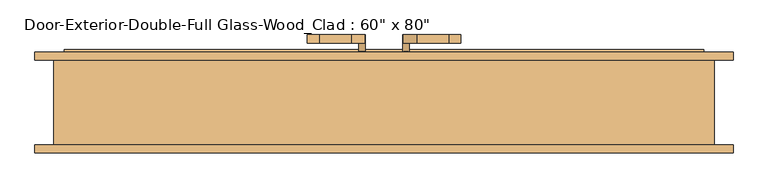
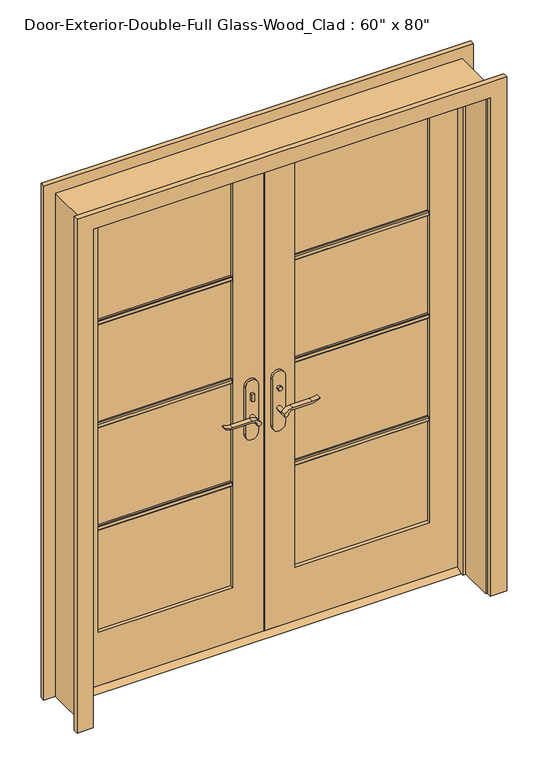
"""IFC4 building model written with IfcOpenShell, lengths in millimetres: door geometry."""

from ifc_helpers import new_model, si_unit, point, frame, frame_2d, origin, place, context, project, spatial, polyline, circle_curve, trimmed, segment, composite_curve, outline, extrude, faceted_brep, source, transform, mapped, element, save


def door_b03bd389(model_context):
    return source(origin(), model_context, "Body", "SolidModel", [
        extrude(outline(polyline([(63.5, 12.7), (98.425, 12.7), (123.825, 0.0), (38.1, 0.0), (63.5, 12.7)])), frame((-762.0, 0.0, 0.0), z_axis=(1.0, 0.0, 0.0), x_axis=(0.0, 1.0, 0.0)), (0.0, 0.0, 1.0), 1524.0),
        extrude(outline(polyline([(-47.4019111, 43.5), (-57.4019111, 43.5), (-57.4019111, 53.5), (-47.4019111, 53.5), (-47.4019111, 43.5)])), frame((0.0, 0.0, 981.9), z_axis=(0.0, 0.0, 1.0), x_axis=(1.0, 0.0, 0.0)), (0.0, 0.0, 1.0), 30.0),
        extrude(outline(composite_curve([segment(trimmed(circle_curve(frame_2d((996.9, -52.4019111)), 8.0), [point((996.9, -60.4019111))], [point((996.9, -44.4019111))], False, "CARTESIAN"), True, "CONTINUOUS"), segment(trimmed(circle_curve(frame_2d((996.9, -52.4019111)), 8.0), [point((996.9, -44.4019111))], [point((996.9, -60.4019111))], False, "CARTESIAN"), True, "CONTINUOUS")], self_intersect=False)), frame((0.0, 108.425, 0.0), z_axis=(0.0, 1.0, 0.0), x_axis=(0.0, 0.0, 1.0)), (0.0, 0.0, 1.0), 10.0),
        extrude(outline(composite_curve([segment(trimmed(circle_curve(frame_2d((897.1555521, -76.0694241)), 37.2832219), [point((919.0523287, -45.8937749))], [point((934.4, -77.7693445))], False, "CARTESIAN"), True, "CONTINUOUS"), segment(polyline([(934.4, -77.7693445), (934.4, -154.045502)]), True, "CONTINUOUS"), segment(trimmed(circle_curve(frame_2d((1017.6850638, -153.9791202)), 83.2850902), [point((934.4, -154.045502))], [point((939.4, -182.4019111))], True, "CARTESIAN"), True, "CONTINUOUS"), segment(polyline([(939.4, -182.4019111), (936.6135558, -182.4019111)]), True, "CONTINUOUS"), segment(trimmed(circle_curve(frame_2d((986.6709207, -150.4622499)), 59.3791355), [point((936.6135558, -182.4019111))], [point((927.4, -154.045502))], False, "CARTESIAN"), True, "CONTINUOUS"), segment(polyline([(927.4, -154.045502), (927.4, -77.7881013)]), True, "CONTINUOUS"), segment(trimmed(circle_curve(frame_2d((909.2738613, -77.7881013)), 18.1261387), [point((927.4, -77.7881013))], [point((914.4, -60.4019111))], True, "CARTESIAN"), True, "CONTINUOUS"), segment(trimmed(circle_curve(frame_2d((914.4, -52.4019111)), 8.0), [point((914.4, -60.4019111))], [point((919.0523287, -45.8937749))], False, "CARTESIAN"), True, "CONTINUOUS")], self_intersect=False)), frame((0.0, 3.5, 0.0), z_axis=(0.0, 1.0, 0.0), x_axis=(0.0, 0.0, 1.0)), (0.0, 0.0, 1.0), 20.0),
        extrude(outline(composite_curve([segment(trimmed(circle_curve(frame_2d((914.4, -52.4019111)), 8.0), [point((914.3999903, -60.4019111))], [point((919.0523287, -45.8937749))], False, "CARTESIAN"), True, "CONTINUOUS"), segment(trimmed(circle_curve(frame_2d((897.1555521, -76.0694241)), 37.2832219), [point((919.0523287, -45.8937749))], [point((934.4, -77.7693445))], False, "CARTESIAN"), True, "CONTINUOUS"), segment(polyline([(934.4, -77.7693445), (934.4, -154.045502)]), True, "CONTINUOUS"), segment(trimmed(circle_curve(frame_2d((1017.6850638, -153.9791202)), 83.2850902), [point((934.4, -154.045502))], [point((939.4, -182.4019111))], True, "CARTESIAN"), True, "CONTINUOUS"), segment(polyline([(939.4, -182.4019111), (936.6135558, -182.4019111)]), True, "CONTINUOUS"), segment(trimmed(circle_curve(frame_2d((986.6709207, -150.4622499)), 59.3791355), [point((936.6135558, -182.4019111))], [point((927.4, -154.045502))], False, "CARTESIAN"), True, "CONTINUOUS"), segment(polyline([(927.4, -154.045502), (927.4, -77.788099)]), True, "CONTINUOUS"), segment(trimmed(circle_curve(frame_2d((909.2738682, -77.788099)), 18.1261318), [point((927.4, -77.788099))], [point((914.3999903, -60.4019111))], True, "CARTESIAN"), True, "CONTINUOUS")], self_intersect=False)), frame((0.0, 138.425, 0.0), z_axis=(0.0, 1.0, 0.0), x_axis=(0.0, 0.0, 1.0)), (0.0, 0.0, 1.0), 20.0),
        extrude(outline(composite_curve([segment(trimmed(circle_curve(frame_2d((914.4, -52.4019111)), 8.0), [point((914.4, -60.4019111))], [point((914.4, -44.4019111))], False, "CARTESIAN"), True, "CONTINUOUS"), segment(trimmed(circle_curve(frame_2d((914.4, -52.4019111)), 8.0), [point((914.4, -44.4019111))], [point((914.4, -60.4019111))], False, "CARTESIAN"), True, "CONTINUOUS")], self_intersect=False)), frame((0.0, 23.5, 0.0), z_axis=(0.0, 1.0, 0.0), x_axis=(0.0, 0.0, 1.0)), (0.0, 0.0, 1.0), 30.0),
        extrude(outline(composite_curve([segment(trimmed(circle_curve(frame_2d((914.4, -52.4019111)), 8.0), [point((914.4, -60.4019111))], [point((914.4, -44.4019111))], False, "CARTESIAN"), True, "CONTINUOUS"), segment(trimmed(circle_curve(frame_2d((914.4, -52.4019111)), 8.0), [point((914.4, -44.4019111))], [point((914.4, -60.4019111))], False, "CARTESIAN"), True, "CONTINUOUS")], self_intersect=False)), frame((0.0, 108.425, 0.0), z_axis=(0.0, 1.0, 0.0), x_axis=(0.0, 0.0, 1.0)), (0.0, 0.0, 1.0), 30.0),
        extrude(outline(composite_curve([segment(polyline([(844.4, -27.4019111), (1039.4, -27.4019111)]), True, "CONTINUOUS"), segment(trimmed(circle_curve(frame_2d((1039.4, -52.4019111)), 25.0), [point((1039.4, -27.4019111))], [point((1039.4, -77.4019111))], False, "CARTESIAN"), True, "CONTINUOUS"), segment(polyline([(1039.4, -77.4019111), (844.4, -77.4019111)]), True, "CONTINUOUS"), segment(trimmed(circle_curve(frame_2d((844.4, -52.4019111)), 25.0), [point((844.4, -77.4019111))], [point((844.4, -27.4019111))], False, "CARTESIAN"), True, "CONTINUOUS")], self_intersect=False)), frame((0.0, 53.5, 0.0), z_axis=(0.0, 1.0, 0.0), x_axis=(0.0, 0.0, 1.0)), (0.0, 0.0, 1.0), 10.0),
        extrude(outline(composite_curve([segment(polyline([(844.4, -27.4019111), (1039.4, -27.4019111)]), True, "CONTINUOUS"), segment(trimmed(circle_curve(frame_2d((1039.4, -52.4019111)), 25.0), [point((1039.4, -27.4019111))], [point((1039.4, -77.4019111))], False, "CARTESIAN"), True, "CONTINUOUS"), segment(polyline([(1039.4, -77.4019111), (844.4, -77.4019111)]), True, "CONTINUOUS"), segment(trimmed(circle_curve(frame_2d((844.4, -52.4019111)), 25.0), [point((844.4, -77.4019111))], [point((844.4, -27.4019111))], False, "CARTESIAN"), True, "CONTINUOUS")], self_intersect=False)), frame((0.0, 98.425, 0.0), z_axis=(0.0, 1.0, 0.0), x_axis=(0.0, 0.0, 1.0)), (0.0, 0.0, 1.0), 10.0),
        extrude(outline(polyline([(47.3875, 118.425), (57.3875, 118.425), (57.3875, 108.425), (47.3875, 108.425), (47.3875, 118.425)])), frame((0.0, 0.0, 981.9), z_axis=(0.0, 0.0, 1.0), x_axis=(1.0, 0.0, 0.0)), (0.0, 0.0, 1.0), 30.0),
        extrude(outline(composite_curve([segment(trimmed(circle_curve(frame_2d((996.9, 52.3875)), 8.0), [point((996.9, 60.3875))], [point((996.9, 44.3875))], False, "CARTESIAN"), True, "CONTINUOUS"), segment(trimmed(circle_curve(frame_2d((996.9, 52.3875)), 8.0), [point((996.9, 44.3875))], [point((996.9, 60.3875))], False, "CARTESIAN"), True, "CONTINUOUS")], self_intersect=False)), frame((0.0, 43.5, 0.0), z_axis=(0.0, 1.0, 0.0), x_axis=(0.0, 0.0, 1.0)), (0.0, 0.0, 1.0), 10.0),
        extrude(outline(composite_curve([segment(trimmed(circle_curve(frame_2d((914.4, 52.3875)), 8.0), [point((919.0523287, 45.8793637))], [point((914.4, 60.3875))], False, "CARTESIAN"), True, "CONTINUOUS"), segment(trimmed(circle_curve(frame_2d((909.2738613, 77.7736901)), 18.1261387), [point((914.4, 60.3875))], [point((927.4, 77.7736901))], True, "CARTESIAN"), True, "CONTINUOUS"), segment(polyline([(927.4, 77.7736901), (927.4, 154.0310909)]), True, "CONTINUOUS"), segment(trimmed(circle_curve(frame_2d((986.6709207, 150.4478388)), 59.3791355), [point((927.4, 154.0310909))], [point((936.6135558, 182.3875))], False, "CARTESIAN"), True, "CONTINUOUS"), segment(polyline([(936.6135558, 182.3875), (939.4, 182.3875)]), True, "CONTINUOUS"), segment(trimmed(circle_curve(frame_2d((1017.6850638, 153.9647091)), 83.2850902), [point((939.4, 182.3875))], [point((934.4, 154.0310909))], True, "CARTESIAN"), True, "CONTINUOUS"), segment(polyline([(934.4, 154.0310909), (934.4, 77.7549333)]), True, "CONTINUOUS"), segment(trimmed(circle_curve(frame_2d((897.1555521, 76.0550129)), 37.2832219), [point((934.4, 77.7549333))], [point((919.0523287, 45.8793637))], False, "CARTESIAN"), True, "CONTINUOUS")], self_intersect=False)), frame((0.0, 138.425, 0.0), z_axis=(0.0, 1.0, 0.0), x_axis=(0.0, 0.0, 1.0)), (0.0, 0.0, 1.0), 20.0),
        extrude(outline(composite_curve([segment(trimmed(circle_curve(frame_2d((909.2738682, 77.7736878)), 18.1261318), [point((914.3999903, 60.3875))], [point((927.4, 77.7736878))], True, "CARTESIAN"), True, "CONTINUOUS"), segment(polyline([(927.4, 77.7736878), (927.4, 154.0310909)]), True, "CONTINUOUS"), segment(trimmed(circle_curve(frame_2d((986.6709207, 150.4478388)), 59.3791355), [point((927.4, 154.0310909))], [point((936.6135558, 182.3875))], False, "CARTESIAN"), True, "CONTINUOUS"), segment(polyline([(936.6135558, 182.3875), (939.4, 182.3875)]), True, "CONTINUOUS"), segment(trimmed(circle_curve(frame_2d((1017.6850638, 153.9647091)), 83.2850902), [point((939.4, 182.3875))], [point((934.4, 154.0310909))], True, "CARTESIAN"), True, "CONTINUOUS"), segment(polyline([(934.4, 154.0310909), (934.4, 77.7549333)]), True, "CONTINUOUS"), segment(trimmed(circle_curve(frame_2d((897.1555521, 76.0550129)), 37.2832219), [point((934.4, 77.7549333))], [point((919.0523287, 45.8793637))], False, "CARTESIAN"), True, "CONTINUOUS"), segment(trimmed(circle_curve(frame_2d((914.4, 52.3875)), 8.0), [point((919.0523287, 45.8793637))], [point((914.3999903, 60.3875))], False, "CARTESIAN"), True, "CONTINUOUS")], self_intersect=False)), frame((0.0, 3.5, 0.0), z_axis=(0.0, 1.0, 0.0), x_axis=(0.0, 0.0, 1.0)), (0.0, 0.0, 1.0), 20.0),
        extrude(outline(composite_curve([segment(trimmed(circle_curve(frame_2d((914.4, 52.3875)), 8.0), [point((914.4, 60.3875))], [point((914.4, 44.3875))], False, "CARTESIAN"), True, "CONTINUOUS"), segment(trimmed(circle_curve(frame_2d((914.4, 52.3875)), 8.0), [point((914.4, 44.3875))], [point((914.4, 60.3875))], False, "CARTESIAN"), True, "CONTINUOUS")], self_intersect=False)), frame((0.0, 108.425, 0.0), z_axis=(0.0, 1.0, 0.0), x_axis=(0.0, 0.0, 1.0)), (0.0, 0.0, 1.0), 30.0),
        extrude(outline(composite_curve([segment(trimmed(circle_curve(frame_2d((914.4, 52.3875)), 8.0), [point((914.4, 60.3875))], [point((914.4, 44.3875))], False, "CARTESIAN"), True, "CONTINUOUS"), segment(trimmed(circle_curve(frame_2d((914.4, 52.3875)), 8.0), [point((914.4, 44.3875))], [point((914.4, 60.3875))], False, "CARTESIAN"), True, "CONTINUOUS")], self_intersect=False)), frame((0.0, 23.5, 0.0), z_axis=(0.0, 1.0, 0.0), x_axis=(0.0, 0.0, 1.0)), (0.0, 0.0, 1.0), 30.0),
        extrude(outline(composite_curve([segment(trimmed(circle_curve(frame_2d((844.4, 52.3875)), 25.0), [point((844.4, 27.3875))], [point((844.4, 77.3875))], False, "CARTESIAN"), True, "CONTINUOUS"), segment(polyline([(844.4, 77.3875), (1039.4, 77.3875)]), True, "CONTINUOUS"), segment(trimmed(circle_curve(frame_2d((1039.4, 52.3875)), 25.0), [point((1039.4, 77.3875))], [point((1039.4, 27.3875))], False, "CARTESIAN"), True, "CONTINUOUS"), segment(polyline([(1039.4, 27.3875), (844.4, 27.3875)]), True, "CONTINUOUS")], self_intersect=False)), frame((0.0, 98.425, 0.0), z_axis=(0.0, 1.0, 0.0), x_axis=(0.0, 0.0, 1.0)), (0.0, 0.0, 1.0), 10.0),
        extrude(outline(composite_curve([segment(trimmed(circle_curve(frame_2d((844.4, 52.3875)), 25.0), [point((844.4, 27.3875))], [point((844.4, 77.3875))], False, "CARTESIAN"), True, "CONTINUOUS"), segment(polyline([(844.4, 77.3875), (1039.4, 77.3875)]), True, "CONTINUOUS"), segment(trimmed(circle_curve(frame_2d((1039.4, 52.3875)), 25.0), [point((1039.4, 77.3875))], [point((1039.4, 27.3875))], False, "CARTESIAN"), True, "CONTINUOUS"), segment(polyline([(1039.4, 27.3875), (844.4, 27.3875)]), True, "CONTINUOUS")], self_intersect=False)), frame((0.0, 53.5, 0.0), z_axis=(0.0, 1.0, 0.0), x_axis=(0.0, 0.0, 1.0)), (0.0, 0.0, 1.0), 10.0),
        extrude(outline(polyline([(77.47, 1502.171875), (77.47, 1483.121875), (71.12, 1483.121875), (67.945, 1486.296875), (67.945, 1498.996875), (71.12, 1502.171875), (77.47, 1502.171875)])), frame((120.65, 0.0, 0.0), z_axis=(1.0, 0.0, 0.0), x_axis=(0.0, 1.0, 0.0)), (0.0, 0.0, 1.0), 520.7),
        extrude(outline(polyline([(77.47, 1081.88125), (77.47, 1062.83125), (71.12, 1062.83125), (67.945, 1066.00625), (67.945, 1078.70625), (71.12, 1081.88125), (77.47, 1081.88125)])), frame((120.65, 0.0, 0.0), z_axis=(1.0, 0.0, 0.0), x_axis=(0.0, 1.0, 0.0)), (0.0, 0.0, 1.0), 520.7),
        extrude(outline(polyline([(77.47, 661.590625), (77.47, 642.540625), (71.12, 642.540625), (67.945, 645.715625), (67.945, 658.415625), (71.12, 661.590625), (77.47, 661.590625)])), frame((120.65, 0.0, 0.0), z_axis=(1.0, 0.0, 0.0), x_axis=(0.0, 1.0, 0.0)), (0.0, 0.0, 1.0), 520.7),
        extrude(outline(polyline([(84.455, 1502.171875), (90.805, 1502.171875), (93.98, 1498.996875), (93.98, 1486.296875), (90.805, 1483.121875), (84.455, 1483.121875), (84.455, 1502.171875)])), frame((-641.35, 0.0, 0.0), z_axis=(1.0, 0.0, 0.0), x_axis=(0.0, 1.0, 0.0)), (0.0, 0.0, 1.0), 520.7),
        extrude(outline(polyline([(84.455, 1081.88125), (90.805, 1081.88125), (93.98, 1078.70625), (93.98, 1066.00625), (90.805, 1062.83125), (84.455, 1062.83125), (84.455, 1081.88125)])), frame((-641.35, 0.0, 0.0), z_axis=(1.0, 0.0, 0.0), x_axis=(0.0, 1.0, 0.0)), (0.0, 0.0, 1.0), 520.7),
        extrude(outline(polyline([(84.455, 661.590625), (90.805, 661.590625), (93.98, 658.415625), (93.98, 645.715625), (90.805, 642.540625), (84.455, 642.540625), (84.455, 661.590625)])), frame((-641.35, 0.0, 0.0), z_axis=(1.0, 0.0, 0.0), x_axis=(0.0, 1.0, 0.0)), (0.0, 0.0, 1.0), 520.7),
        extrude(outline(polyline([(84.455, 1502.171875), (90.805, 1502.171875), (93.98, 1498.996875), (93.98, 1486.296875), (90.805, 1483.121875), (84.455, 1483.121875), (84.455, 1502.171875)])), frame((120.65, 0.0, 0.0), z_axis=(1.0, 0.0, 0.0), x_axis=(0.0, 1.0, 0.0)), (0.0, 0.0, 1.0), 520.7),
        extrude(outline(polyline([(84.455, 1081.88125), (90.805, 1081.88125), (93.98, 1078.70625), (93.98, 1066.00625), (90.805, 1062.83125), (84.455, 1062.83125), (84.455, 1081.88125)])), frame((120.65, 0.0, 0.0), z_axis=(1.0, 0.0, 0.0), x_axis=(0.0, 1.0, 0.0)), (0.0, 0.0, 1.0), 520.7),
        extrude(outline(polyline([(84.455, 661.590625), (90.805, 661.590625), (93.98, 658.415625), (93.98, 645.715625), (90.805, 642.540625), (84.455, 642.540625), (84.455, 661.590625)])), frame((120.65, 0.0, 0.0), z_axis=(1.0, 0.0, 0.0), x_axis=(0.0, 1.0, 0.0)), (0.0, 0.0, 1.0), 520.7),
        extrude(outline(polyline([(77.47, 1502.171875), (77.47, 1483.121875), (71.12, 1483.121875), (67.945, 1486.296875), (67.945, 1498.996875), (71.12, 1502.171875), (77.47, 1502.171875)])), frame((-641.35, 0.0, 0.0), z_axis=(1.0, 0.0, 0.0), x_axis=(0.0, 1.0, 0.0)), (0.0, 0.0, 1.0), 520.7),
        extrude(outline(polyline([(77.47, 1081.88125), (77.47, 1062.83125), (71.12, 1062.83125), (67.945, 1066.00625), (67.945, 1078.70625), (71.12, 1081.88125), (77.47, 1081.88125)])), frame((-641.35, 0.0, 0.0), z_axis=(1.0, 0.0, 0.0), x_axis=(0.0, 1.0, 0.0)), (0.0, 0.0, 1.0), 520.7),
        extrude(outline(polyline([(77.47, 661.590625), (77.47, 642.540625), (71.12, 642.540625), (67.945, 645.715625), (67.945, 658.415625), (71.12, 661.590625), (77.47, 661.590625)])), frame((-641.35, 0.0, 0.0), z_axis=(1.0, 0.0, 0.0), x_axis=(0.0, 1.0, 0.0)), (0.0, 0.0, 1.0), 520.7),
        extrude(outline(polyline([(0.0, 768.35), (0.0, 831.85), (2101.85, 831.85), (2101.85, -831.85), (0.0, -831.85), (0.0, -768.35), (2038.35, -768.35), (2038.35, 768.35), (0.0, 768.35)])), frame((0.0, 98.425, 0.0), z_axis=(0.0, 1.0, 0.0), x_axis=(0.0, 0.0, 1.0)), (0.0, 0.0, 1.0), 19.05),
        extrude(outline(polyline([(0.0, 768.35), (0.0, 831.85), (2101.85, 831.85), (2101.85, -831.85), (0.0, -831.85), (0.0, -768.35), (2038.35, -768.35), (2038.35, 768.35), (0.0, 768.35)])), frame((0.0, -123.825, 0.0), z_axis=(0.0, 1.0, 0.0), x_axis=(0.0, 0.0, 1.0)), (0.0, 0.0, 1.0), 19.05),
        extrude(outline(polyline([(12.7, 762.0), (2032.0, 762.0), (2032.0, 1.5875), (12.7, 1.5875), (12.7, 762.0)]), holes=[polyline([(1912.9375, 120.65), (1912.9375, 641.35), (231.775, 641.35), (231.775, 120.65), (1912.9375, 120.65)])]), frame((0.0, 63.5, 0.0), z_axis=(0.0, 1.0, 0.0), x_axis=(0.0, 0.0, 1.0)), (0.0, 0.0, 1.0), 34.925),
        extrude(outline(polyline([(2032.0, -762.0), (12.7, -762.0), (12.7, -1.6019111), (2032.0, -1.6019111), (2032.0, -762.0)]), holes=[polyline([(231.775, -641.35), (1912.9375, -641.35), (1912.9375, -120.65), (231.775, -120.65), (231.775, -641.35)])]), frame((0.0, 63.5, 0.0), z_axis=(0.0, 1.0, 0.0), x_axis=(0.0, 0.0, 1.0)), (0.0, 0.0, 1.0), 34.925),
        faceted_brep([(787.4, 98.425, 0.0), (787.4, -104.775, 0.0), (762.0, -104.775, 0.0), (762.0, 28.575, 0.0), (749.3, 28.575, 0.0), (749.3, 63.5, 0.0), (762.0, 63.5, 0.0), (762.0, 98.425, 0.0), (787.4, 98.425, 2057.4), (787.4, -104.775, 2057.4), (-787.4, -104.775, 2057.4), (-787.4, -104.775, 0.0), (-762.0, -104.775, 0.0), (-762.0, -104.775, 2032.0), (762.0, -104.775, 2032.0), (762.0, 28.575, 2032.0), (-762.0, 28.575, 2032.0), (-762.0, 28.575, 0.0), (-749.3, 28.575, 0.0), (-749.3, 28.575, 2019.3), (749.3, 28.575, 2019.3), (749.3, 63.5, 2019.3), (1.5875, 63.5, 2019.3), (-1.6019111, 63.5, 2019.3), (-749.3, 63.5, 2019.3), (-749.3, 63.5, 0.0), (-762.0, 63.5, 0.0), (-762.0, 63.5, 2032.0), (-1.6019111, 63.5, 2032.0), (1.5875, 63.5, 2032.0), (762.0, 63.5, 2032.0), (762.0, 98.425, 2032.0), (1.5875, 98.425, 2032.0), (-1.6019111, 98.425, 2032.0), (-762.0, 98.425, 2032.0), (-762.0, 98.425, 0.0), (-787.4, 98.425, 0.0), (-787.4, 98.425, 2057.4)], [[[0, 1, 2, 3, 4, 5, 6, 7]], [[1, 0, 8, 9]], [[2, 1, 9, 10, 11, 12, 13, 14]], [[3, 2, 14, 15]], [[4, 3, 15, 16, 17, 18, 19, 20]], [[5, 4, 20, 21]], [[6, 5, 21, 22, 23, 24, 25, 26, 27, 28, 29, 30]], [[7, 6, 30, 31]], [[0, 7, 31, 32, 33, 34, 35, 36, 37, 8]], [[9, 8, 37, 10]], [[14, 13, 16, 15]], [[20, 19, 24, 23, 22, 21]], [[31, 30, 29, 28, 27, 34, 33, 32]], [[12, 11, 36, 35, 26, 25, 18, 17]], [[11, 10, 37, 36]], [[13, 12, 17, 16]], [[19, 18, 25, 24]], [[27, 26, 35, 34]]]),
        extrude(outline(polyline([(641.35, 77.47), (120.65, 77.47), (120.65, 84.455), (641.35, 84.455), (641.35, 77.47)])), frame((0.0, 0.0, 231.775), z_axis=(0.0, 0.0, 1.0), x_axis=(1.0, 0.0, 0.0)), (0.0, 0.0, 1.0), 1681.1625),
        extrude(outline(polyline([(-120.65, 77.47), (-641.35, 77.47), (-641.35, 84.455), (-120.65, 84.455), (-120.65, 77.47)])), frame((0.0, 0.0, 231.775), z_axis=(0.0, 0.0, 1.0), x_axis=(1.0, 0.0, 0.0)), (0.0, 0.0, 1.0), 1681.1625),
    ])


if __name__ == "__main__":
    model = new_model("IFC4")
    model_context = context("Model", 3, world=origin())
    ifc_project = project(units=[si_unit("LENGTHUNIT", "METRE", prefix="MILLI")], contexts=[model_context])
    site = spatial("IfcSite", under=ifc_project)
    building = spatial("IfcBuilding", under=site)
    placement = place(None, origin())
    door_shape = door_b03bd389(model_context)
    element("IfcDoor", 1, ObjectType="Door-Exterior-Double-Full Glass-Wood_Clad : 60\" x 80\"", at=placement, inside=building, context=model_context, shape_type="MappedRepresentation", body=[
        mapped(door_shape, transform((0.0, 0.0, 0.0), x_axis=(1.0, 0.0, 0.0), y_axis=(0.0, 1.0, 0.0), z_axis=(0.0, 0.0, 1.0))),
    ])
    save(model, "model.ifc")

# Revit data of these elements
# Type "Door-Exterior-Double-Full Glass-Wood_Clad : 60\" x 80\""
#   Type Mark = "10"
#   Assembly Code = "B2030100"
#   Analytic Construction = "French door, wood frame with double glass"
#   Top Rail = 0' - 4 11/16"
#   Threshold Offset [instance default] = 0' - 0 1/2"
#   Thickness = 0' - 1 3/8"
#   Thermal Resistance (R) = 1.9158 (h·ft²·°F)/BTU
#   Swing Angle [instance default] = 90.00°
#   Stiles = 0' - 4 3/4"
#   Rough Width = 5' - 2"
#   Rough Height = 6' - 9"
#   Panel Width = 2' - 6"
#   Door Offset [instance default] = 0' - 0"
#   Height = 6' - 8"
#   Width = 5' - 0"
#   Heat Transfer Coefficient (U) = 0.5220 BTU/(h·ft²·°F)
#   Bottom Rail = 0' - 9 1/8"
#   Exterior Trim [instance default] = yes
#   Threshold [instance default] = yes
#   Show Grill [instance default] = yes
#   Function = 1
#   Trim Material = Cherry
#   Threshold Material = Cherry
#   Panel Material = Cherry
#   Glazing = Glass
#   Frame Material = Cherry
#   Door Handle Material = Aluminum
#   Visual Light Transmittance = 0
#   Solar Heat Gain Coefficient = 0
#   Wall Closure = (empty or 0)
#   Construction Type = (empty or 0)
# Element 1 (IfcDoor, "Door-Exterior-Double-Full Glass-Wood_Clad : 60\" x 80\"")
#   Materials on its faces: "Cherry", "Aluminum", "Glass"
# Materials
#   "Cherry": class "Wood", colour RGB 226 177 128, transparency 0, Description = "Prunus Serotina", Cost = 0
#   "Glass": class "Glass", colour RGB 0 128 192, transparency 0.75, Description = "Soda Lime Glass", Cost = 0
#   "Aluminum": class "Metal", colour RGB 247 247 247, transparency 0, Description = "Aluminum 6061", Cost = 0
